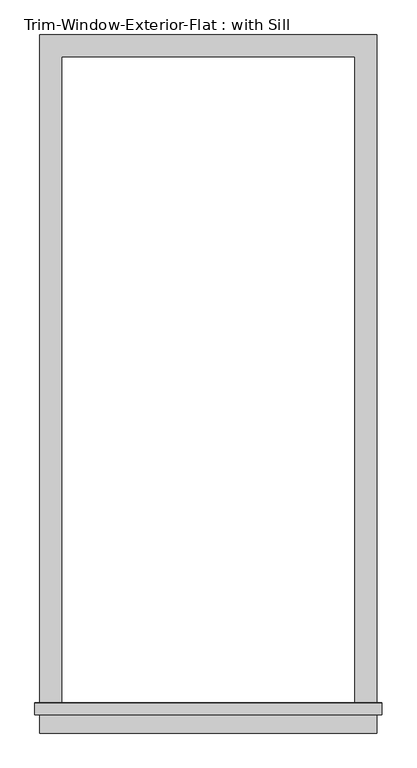
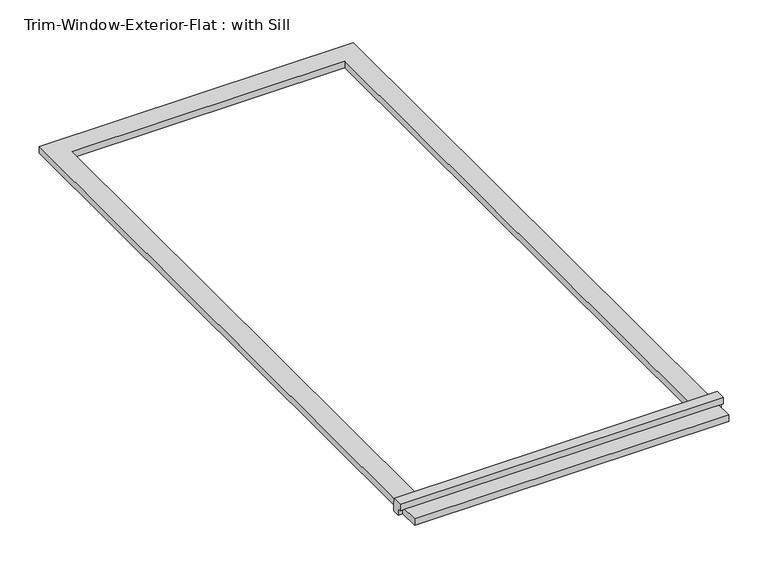
"""IFC4 building model written with IfcOpenShell, lengths in millimetres: proxy geometry, Trim-Window-Exterior-Flat : with Sill."""

from ifc_helpers import new_model, si_unit, frame, origin, origin_with_axes, place, context, project, spatial, polyline, outline, extrude, source, transform, mapped, element, save


def trim_window_exterior_flat_with_sill_8633aa7b(model_context):
    return source(origin(), model_context, "Body", "SweptSolid", [
        extrude(outline(polyline([(438.15, -1698.5823709), (438.15, -1755.7323709), (-438.15, -1755.7323709), (-438.15, -1698.5823709), (438.15, -1698.5823709)])), origin_with_axes(), (0.0, 0.0, 1.0), 19.05),
        extrude(outline(polyline([(-1708.15, 38.1), (-1678.8580645, 38.1), (-1676.4, 19.05), (-1676.4, 0.0), (-1698.5823709, 0.0), (-1698.5823709, 19.05), (-1708.15, 19.05), (-1708.15, 38.1)])), frame((-450.85, 0.0, 0.0), z_axis=(1.0, 0.0, 0.0), x_axis=(0.0, 1.0, 0.0)), (0.0, 0.0, 1.0), 901.7),
        extrude(outline(polyline([(-438.15, 57.15), (438.15, 57.15), (438.15, -1676.4), (381.0, -1676.4), (381.0, 0.0), (-381.0, 0.0), (-381.0, -1676.4), (-438.15, -1676.4), (-438.15, 57.15)])), origin_with_axes(), (0.0, 0.0, 1.0), 19.05),
    ])


if __name__ == "__main__":
    model = new_model("IFC4")
    model_context = context("Model", 3, world=origin())
    ifc_project = project(units=[si_unit("LENGTHUNIT", "METRE", prefix="MILLI")], contexts=[model_context])
    site = spatial("IfcSite", under=ifc_project)
    building = spatial("IfcBuilding", under=site)
    placement = place(None, origin())
    trim_window_exterior_flat_with_sill_shape = trim_window_exterior_flat_with_sill_8633aa7b(model_context)
    element("IfcBuildingElementProxy", 1, Name="Trim-Window-Exterior-Flat : with Sill", ObjectType="Trim-Window-Exterior-Flat : with Sill", at=placement, inside=building, context=model_context, shape_type="MappedRepresentation", body=[
        mapped(trim_window_exterior_flat_with_sill_shape, transform((0.0, 0.0, 0.0), x_axis=(1.0, 0.0, 0.0), y_axis=(0.0, 1.0, 0.0), z_axis=(0.0, 0.0, 1.0))),
    ])
    save(model, "model.ifc")

# Revit data of these elements
# Type "Trim-Window-Exterior-Flat : with Sill"
#   Trim Width = 0' - 2 1/4"
#   Trim Thickness_Picture Frame = 0' - 1 1/4"
#   Trim Thickness_with Sill = 0' - 0 3/4"
#   Sill Thickness = 0' - 1 1/4"
#   Opening Width [instance default] = 2' - 0"
#   Opening Height [instance default] = 3' - 0"
#   Default Elevation = 4' - 0"
#   Sill = yes
#   Picture Frame = no
#   Trim Material [instance default] = none
# Element 1 (IfcBuildingElementProxy, "Trim-Window-Exterior-Flat : with Sill")
#   Opening Width = 2' - 6"
#   Opening Height = 5' - 6"
#   Trim Material = Clad - White
#   Materials on its faces: "Clad - White"
# Materials
#   "Clad - White": class "Wood", colour RGB 242 242 238, transparency 0, Cost = 0
